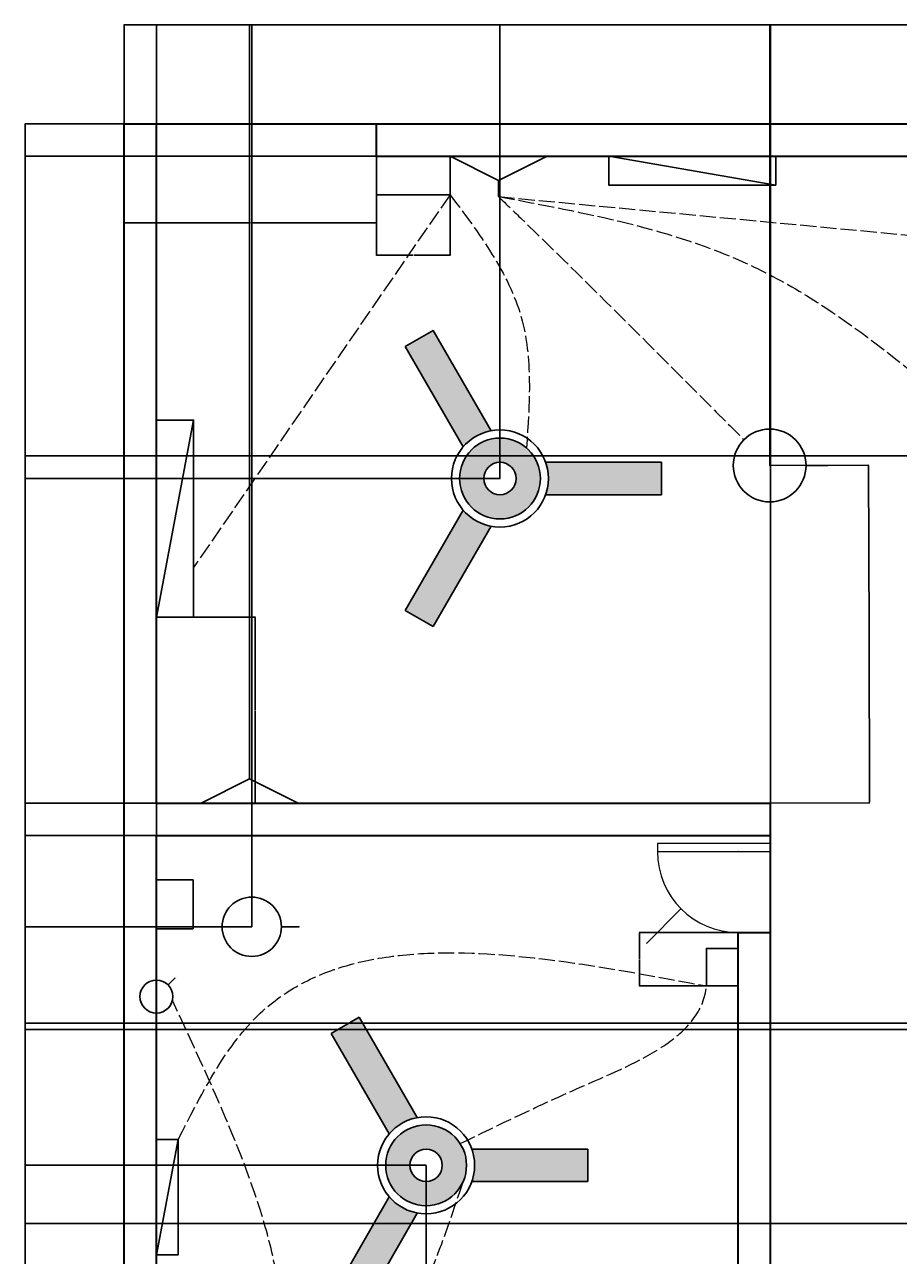
# Model space of a CAD drawing. Units: inches. Extents: x 2034 to 3646, y 962 to 2549.
# Tile 2 of 4: x 2034 to 2683, y 1636 to 2549. Entities that reach past the tile are written whole.
import ezdxf

# ---------------------------------------------------------------- set-up
doc = ezdxf.new("R2010")
doc.units = ezdxf.units.IN
doc.linetypes.add('ACAD_ISO02W100', pattern=[15, 12, -3])
for name, color, linetype, lineweight in [('A-ANNO-DIMS', 2, 'Continuous', 18), ('E-EQPM-FANS', 7, 'Continuous', 30), ('E-LITE-CTRL', 7, 'Continuous', 25), ('E-LITE-FIXT', 7, 'Continuous', 25), ('E-POWR-DEVC', 7, 'Continuous', 25)]:
    doc.layers.add(name, color=color, linetype=linetype, lineweight=lineweight)
for name, color, linetype, lineweight, true_color in [('A-DOOR', 203, 'Continuous', 18, 0xa780c2), ('A-WALL', 203, 'Continuous', 35, 0xa780c2), ('E-LITE-WIRE', 103, 'ACAD_ISO02W100', 18, 0x6dc08b)]:
    doc.layers.add(name, color=color, linetype=linetype, lineweight=lineweight, true_color=true_color)
doc.styles.get("Standard").update_dxf_attribs({"font": 'arial.ttf'})
doc.dimstyles.get("Standard").update_dxf_attribs({"dimtxt": 0.18, "dimasz": 0.18, "dimexe": 0.18, "dimexo": 0.0625, "dimgap": 0.09, "dimtad": 0, "dimtih": 1, "dimtoh": 1, "dimdec": 4, "dimzin": 0, "dimdsep": 46, "dimtxsty": 'Standard', "dimcen": 0.09, "dimadec": 0, "dimazin": 0, "dimtfac": 1, "dimtdec": 4, "dimtofl": 0, "dimtmove": 0, "dimatfit": 3, "dimfxl": 1, "dimtolj": 1, "dimtzin": 0, "dimarcsym": 0})

# ---------------------------------------------------------------- blocks, each defined once
blk = doc.blocks.new('CEILING-FAN-3-BLADE')
h = blk.add_hatch(color=256)
h.dxf.hatch_style = 1
h.paths.add_polyline_path([(-49.61, 109.92), (-70.39, 97.92), (-27.36, 23.39, -0.171573), (-6.58, 35.39)])
h = blk.add_hatch(color=256)
h.dxf.hatch_style = 1
h.paths.add_polyline_path([(-30, 0, 1), (30, 0, 1)])
h.paths.add_polyline_path([(12, 0, -1), (-12, 0, -1)], flags=16)
h = blk.add_hatch(color=256)
h.dxf.hatch_style = 1
h.paths.add_polyline_path([(120, 12), (33.94, 12, -0.085164), (36, 0, -0.085164), (33.94, -12), (120, -12)])
h = blk.add_hatch(color=256)
h.dxf.hatch_style = 1
h.paths.add_polyline_path([(-6.58, -35.39, -0.171573), (-27.36, -23.39), (-70.39, -97.92), (-49.61, -109.92)])
for p, q in [((-70.39, 97.92), (-49.61, 109.92)), ((-49.61, 109.92), (-6.58, 35.39)), ((-27.36, 23.39), (-70.39, 97.92)), ((33.94, 12), (120, 12)), ((120, 12), (120, -12)), ((120, -12), (33.94, -12)), ((-70.39, -97.92), (-27.36, -23.39)), ((-6.58, -35.39), (-49.61, -109.92)), ((-49.61, -109.92), (-70.39, -97.92))]:
    blk.add_line(p, q)
for radius in [36, 30, 12]:
    blk.add_circle((0, 0), radius)
blk = doc.blocks.new('WALL-DEVICE-TRIANGLE')
for p, q in [((-36, 0), (36, 0)), ((0, -18), (-36, 0)), ((36, 0), (0, -18)), ((0, -18), (0, -30))]:
    blk.add_line(p, q)
blk = doc.blocks.new('*D4')
at = {"layer": 'A-ANNO-DIMS', "color": 0, "lineweight": -2, "transparency": 16777216}
for p, q in [((2108.2, 2475.7), (2108.2, 2549.27)), ((2108.38, 2549.09), (2839.85, 2549.09)), ((3572.02, 2549.09), (2840.55, 2549.09)), ((3572.2, 2475.7), (3572.2, 2549.27))]:
    blk.add_line(p, q, dxfattribs=at)
at = {"layer": 'A-ANNO-DIMS', "color": 0, "transparency": 16777216}
for points in [[(2108.38, 2549.12), (2108.38, 2549.06), (2108.2, 2549.09)], [(3572.02, 2549.12), (3572.02, 2549.06), (3572.2, 2549.09)]]:
    blk.add_solid(points, dxfattribs=at)
at = {"layer": 'Defpoints', "color": 0, "transparency": 16777216}
for p in [(3572.2, 2549.09), (2108.2, 2475.64), (3572.2, 2475.64)]:
    blk.add_point(p, dxfattribs=at)
at = {"layer": 'A-ANNO-DIMS', "color": 0, "transparency": 16777216, "insert": (2840.2, 2549.09), "char_height": 0.18, "attachment_point": 5}
blk.add_mtext('\\A1;1464', dxfattribs=at)
blk = doc.blocks.new('*D5')
at = {"layer": 'A-ANNO-DIMS', "color": 0, "lineweight": -2, "transparency": 16777216}
for p, q in [((2108.14, 2475.64), (2034.57, 2475.64)), ((2034.75, 2475.46), (2034.75, 1755.82)), ((2034.75, 1035.82), (2034.75, 1755.46)), ((2682.26, 1035.64), (2034.57, 1035.64))]:
    blk.add_line(p, q, dxfattribs=at)
at = {"layer": 'A-ANNO-DIMS', "color": 0, "transparency": 16777216}
for points in [[(2034.72, 2475.46), (2034.78, 2475.46), (2034.75, 2475.64)], [(2034.72, 1035.82), (2034.78, 1035.82), (2034.75, 1035.64)]]:
    blk.add_solid(points, dxfattribs=at)
at = {"layer": 'Defpoints', "color": 0, "transparency": 16777216}
for p in [(2034.75, 2475.64), (2108.2, 2475.64), (2682.32, 1035.64)]:
    blk.add_point(p, dxfattribs=at)
at = {"layer": 'A-ANNO-DIMS', "color": 0, "transparency": 16777216, "insert": (2034.75, 1755.64), "char_height": 0.18, "attachment_point": 5}
blk.add_mtext('\\A1;1440', dxfattribs=at)
blk = doc.blocks.new('*D14')
at = {"layer": 'A-ANNO-DIMS', "color": 0, "lineweight": -2, "transparency": 16777216}
for p, q in [((2132.14, 2451.64), (2034.57, 2451.64)), ((2034.75, 2451.46), (2034.75, 2211.82)), ((2034.75, 1971.82), (2034.75, 2211.46)), ((2132.14, 1971.64), (2034.57, 1971.64))]:
    blk.add_line(p, q, dxfattribs=at)
at = {"layer": 'A-ANNO-DIMS', "color": 0, "transparency": 16777216}
for points in [[(2034.72, 2451.46), (2034.78, 2451.46), (2034.75, 2451.64)], [(2034.72, 1971.82), (2034.78, 1971.82), (2034.75, 1971.64)]]:
    blk.add_solid(points, dxfattribs=at)
at = {"layer": 'Defpoints', "color": 0, "transparency": 16777216}
for p in [(2034.75, 2451.64), (2132.2, 2451.64), (2132.2, 1971.64)]:
    blk.add_point(p, dxfattribs=at)
at = {"layer": 'A-ANNO-DIMS', "color": 0, "transparency": 16777216, "insert": (2034.75, 2211.64), "char_height": 0.18, "attachment_point": 5}
blk.add_mtext('\\A1;480', dxfattribs=at)
blk = doc.blocks.new('*D15')
at = {"layer": 'A-ANNO-DIMS', "color": 0, "lineweight": -2, "transparency": 16777216}
for p, q in [((2588.2, 1971.7), (2588.2, 2549.27)), ((2588.38, 2549.09), (2705.7, 2549.09)), ((2823.95, 2549.09), (2706.63, 2549.09)), ((2824.13, 1971.7), (2824.13, 2549.27))]:
    blk.add_line(p, q, dxfattribs=at)
at = {"layer": 'A-ANNO-DIMS', "color": 0, "transparency": 16777216}
for points in [[(2588.38, 2549.12), (2588.38, 2549.06), (2588.2, 2549.09)], [(2823.95, 2549.12), (2823.95, 2549.06), (2824.13, 2549.09)]]:
    blk.add_solid(points, dxfattribs=at)
at = {"layer": 'Defpoints', "color": 0, "transparency": 16777216}
for p in [(2824.13, 2549.09), (2588.2, 1971.64), (2824.13, 1971.64)]:
    blk.add_point(p, dxfattribs=at)
at = {"layer": 'A-ANNO-DIMS', "color": 0, "transparency": 16777216, "insert": (2706.16, 2549.09), "char_height": 0.18, "attachment_point": 5}
blk.add_mtext('\\A1;235.93', dxfattribs=at)
blk = doc.blocks.new('*D16')
at = {"layer": 'A-ANNO-DIMS', "color": 0, "lineweight": -2, "transparency": 16777216}
for p, q in [((2588.2, 1635.7), (2588.2, 2549.27)), ((2588.38, 2549.09), (2935.91, 2549.09)), ((3284.02, 2549.09), (2936.49, 2549.09)), ((3284.2, 1635.7), (3284.2, 2549.27))]:
    blk.add_line(p, q, dxfattribs=at)
at = {"layer": 'A-ANNO-DIMS', "color": 0, "transparency": 16777216}
for points in [[(2588.38, 2549.12), (2588.38, 2549.06), (2588.2, 2549.09)], [(3284.02, 2549.12), (3284.02, 2549.06), (3284.2, 2549.09)]]:
    blk.add_solid(points, dxfattribs=at)
at = {"layer": 'Defpoints', "color": 0, "transparency": 16777216}
for p in [(3284.2, 2549.09), (2588.2, 1635.64), (3284.2, 1635.64)]:
    blk.add_point(p, dxfattribs=at)
at = {"layer": 'A-ANNO-DIMS', "color": 0, "transparency": 16777216, "insert": (2936.2, 2549.09), "char_height": 0.18, "attachment_point": 5}
blk.add_mtext('\\A1;696', dxfattribs=at)
blk = doc.blocks.new('*D20')
at = {"layer": 'A-ANNO-DIMS', "color": 0, "lineweight": -2, "transparency": 16777216}
for p, q in [((3300.28, 1803.64), (2034.57, 1803.64)), ((2034.75, 1803.46), (2034.75, 1731.82)), ((2034.75, 1659.82), (2034.75, 1731.46)), ((3300.28, 1659.64), (2034.57, 1659.64))]:
    blk.add_line(p, q, dxfattribs=at)
at = {"layer": 'A-ANNO-DIMS', "color": 0, "transparency": 16777216}
for points in [[(2034.72, 1803.46), (2034.78, 1803.46), (2034.75, 1803.64)], [(2034.72, 1659.82), (2034.78, 1659.82), (2034.75, 1659.64)]]:
    blk.add_solid(points, dxfattribs=at)
at = {"layer": 'Defpoints', "color": 0, "transparency": 16777216}
for p in [(2034.75, 1803.64), (3300.34, 1803.64), (3300.34, 1659.64)]:
    blk.add_point(p, dxfattribs=at)
at = {"layer": 'A-ANNO-DIMS', "color": 0, "transparency": 16777216, "insert": (2034.75, 1731.64), "char_height": 0.18, "attachment_point": 5}
blk.add_mtext('\\A1;144', dxfattribs=at)
blk = doc.blocks.new('*D24')
at = {"layer": 'A-ANNO-DIMS', "color": 0, "lineweight": -2, "transparency": 16777216}
for p, q in [((2132.2, 2255.92), (2132.2, 2549.27)), ((2132.38, 2549.09), (2259.25, 2549.09)), ((2387.05, 2549.09), (2260.18, 2549.09)), ((2387.23, 2212.56), (2387.23, 2549.27))]:
    blk.add_line(p, q, dxfattribs=at)
at = {"layer": 'A-ANNO-DIMS', "color": 0, "transparency": 16777216}
for points in [[(2132.38, 2549.12), (2132.38, 2549.06), (2132.2, 2549.09)], [(2387.05, 2549.12), (2387.05, 2549.06), (2387.23, 2549.09)]]:
    blk.add_solid(points, dxfattribs=at)
at = {"layer": 'Defpoints', "color": 0, "transparency": 16777216}
for p in [(2387.23, 2549.09), (2132.2, 2255.85), (2387.23, 2212.5)]:
    blk.add_point(p, dxfattribs=at)
at = {"layer": 'A-ANNO-DIMS', "color": 0, "transparency": 16777216, "insert": (2259.71, 2549.09), "char_height": 0.18, "attachment_point": 5}
blk.add_mtext('\\A1;255.03', dxfattribs=at)
blk = doc.blocks.new('*D25')
at = {"layer": 'A-ANNO-DIMS', "color": 0, "lineweight": -2, "transparency": 16777216}
for p, q in [((2387.23, 2212.56), (2387.23, 2549.27)), ((2387.41, 2549.09), (2486.88, 2549.09)), ((2587.29, 2549.09), (2487.81, 2549.09)), ((2587.47, 2222.22), (2587.47, 2549.27))]:
    blk.add_line(p, q, dxfattribs=at)
at = {"layer": 'A-ANNO-DIMS', "color": 0, "transparency": 16777216}
for points in [[(2387.41, 2549.12), (2387.41, 2549.06), (2387.23, 2549.09)], [(2587.29, 2549.12), (2587.29, 2549.06), (2587.47, 2549.09)]]:
    blk.add_solid(points, dxfattribs=at)
at = {"layer": 'Defpoints', "color": 0, "transparency": 16777216}
for p in [(2587.47, 2549.09), (2587.47, 2222.15), (2387.23, 2212.5)]:
    blk.add_point(p, dxfattribs=at)
at = {"layer": 'A-ANNO-DIMS', "color": 0, "transparency": 16777216, "insert": (2487.35, 2549.09), "char_height": 0.18, "attachment_point": 5}
blk.add_mtext('\\A1;200.24', dxfattribs=at)
blk = doc.blocks.new('*D26')
at = {"layer": 'A-ANNO-DIMS', "color": 0, "lineweight": -2, "transparency": 16777216}
for p, q in [((2587.47, 2222.22), (2587.47, 2549.27)), ((2587.65, 2549.09), (2679.2, 2549.09)), ((2771.3, 2549.09), (2679.76, 2549.09)), ((2771.48, 2229.49), (2771.48, 2549.27))]:
    blk.add_line(p, q, dxfattribs=at)
at = {"layer": 'A-ANNO-DIMS', "color": 0, "transparency": 16777216}
for points in [[(2587.65, 2549.12), (2587.65, 2549.06), (2587.47, 2549.09)], [(2771.3, 2549.12), (2771.3, 2549.06), (2771.48, 2549.09)]]:
    blk.add_solid(points, dxfattribs=at)
at = {"layer": 'Defpoints', "color": 0, "transparency": 16777216}
for p in [(2771.48, 2549.09), (2771.48, 2229.42), (2587.47, 2222.15)]:
    blk.add_point(p, dxfattribs=at)
at = {"layer": 'A-ANNO-DIMS', "color": 0, "transparency": 16777216, "insert": (2679.48, 2549.09), "char_height": 0.18, "attachment_point": 5}
blk.add_mtext('\\A1;184', dxfattribs=at)
blk = doc.blocks.new('*D27')
at = {"layer": 'A-ANNO-DIMS', "color": 0, "lineweight": -2, "transparency": 16777216}
for p, q in [((2387.17, 2212.5), (2034.57, 2212.5)), ((2034.75, 2212.32), (2034.75, 2092.25)), ((2034.75, 1971.82), (2034.75, 2091.89)), ((2132.14, 1971.64), (2034.57, 1971.64))]:
    blk.add_line(p, q, dxfattribs=at)
at = {"layer": 'A-ANNO-DIMS', "color": 0, "transparency": 16777216}
for points in [[(2034.72, 2212.32), (2034.78, 2212.32), (2034.75, 2212.5)], [(2034.72, 1971.82), (2034.78, 1971.82), (2034.75, 1971.64)]]:
    blk.add_solid(points, dxfattribs=at)
at = {"layer": 'Defpoints', "color": 0, "transparency": 16777216}
for p in [(2034.75, 2212.5), (2387.23, 2212.5), (2132.2, 1971.64)]:
    blk.add_point(p, dxfattribs=at)
at = {"layer": 'A-ANNO-DIMS', "color": 0, "transparency": 16777216, "insert": (2034.75, 2092.07), "char_height": 0.18, "attachment_point": 5}
blk.add_mtext('\\A1;240.86', dxfattribs=at)
blk = doc.blocks.new('*D28')
at = {"layer": 'A-ANNO-DIMS', "color": 0, "lineweight": -2, "transparency": 16777216}
for p, q in [((2785.69, 2451.64), (2034.57, 2451.64)), ((2034.75, 2451.46), (2034.75, 2340.71)), ((2034.75, 2229.6), (2034.75, 2340.35)), ((2771.42, 2229.42), (2034.57, 2229.42))]:
    blk.add_line(p, q, dxfattribs=at)
at = {"layer": 'A-ANNO-DIMS', "color": 0, "transparency": 16777216}
for points in [[(2034.72, 2451.46), (2034.78, 2451.46), (2034.75, 2451.64)], [(2034.72, 2229.6), (2034.78, 2229.6), (2034.75, 2229.42)]]:
    blk.add_solid(points, dxfattribs=at)
at = {"layer": 'Defpoints', "color": 0, "transparency": 16777216}
for p in [(2034.75, 2451.64), (2785.75, 2451.64), (2771.48, 2229.42)]:
    blk.add_point(p, dxfattribs=at)
at = {"layer": 'A-ANNO-DIMS', "color": 0, "transparency": 16777216, "insert": (2034.75, 2340.53), "char_height": 0.18, "attachment_point": 5}
blk.add_mtext('\\A1;222.2', dxfattribs=at)
blk = doc.blocks.new('*D29')
at = {"layer": 'A-ANNO-DIMS', "color": 0, "lineweight": -2, "transparency": 16777216}
for p, q in [((2587.53, 2222.15), (2661.1, 2222.37)), ((2660.92, 2222.19), (2661.28, 2097.29)), ((2661.65, 1972.03), (2661.28, 2096.93)), ((2588.26, 1971.64), (2661.83, 1971.85))]:
    blk.add_line(p, q, dxfattribs=at)
at = {"layer": 'A-ANNO-DIMS', "color": 0, "transparency": 16777216}
for points in [[(2660.95, 2222.19), (2660.89, 2222.19), (2660.92, 2222.37)], [(2661.68, 1972.03), (2661.62, 1972.03), (2661.65, 1971.85)]]:
    blk.add_solid(points, dxfattribs=at)
at = {"layer": 'Defpoints', "color": 0, "transparency": 16777216}
for p in [(2587.47, 2222.15), (2588.2, 1971.64), (2661.65, 1971.85)]:
    blk.add_point(p, dxfattribs=at)
at = {"layer": 'A-ANNO-DIMS', "color": 0, "transparency": 16777216, "insert": (2661.28, 2097.11), "char_height": 0.18, "attachment_point": 5}
blk.add_mtext('\\A1;250.5', dxfattribs=at)
blk = doc.blocks.new('*D30')
at = {"layer": 'A-ANNO-DIMS', "color": 0, "lineweight": -2, "transparency": 16777216}
for p, q in [((2332.44, 1702.82), (2332.44, 962.01)), ((2132.2, 1431.58), (2132.2, 962.01)), ((2132.38, 962.19), (2231.85, 962.19)), ((2332.26, 962.19), (2232.78, 962.19))]:
    blk.add_line(p, q, dxfattribs=at)
at = {"layer": 'A-ANNO-DIMS', "color": 0, "transparency": 16777216}
for points in [[(2132.38, 962.22), (2132.38, 962.16), (2132.2, 962.19)], [(2332.26, 962.22), (2332.26, 962.16), (2332.44, 962.19)]]:
    blk.add_solid(points, dxfattribs=at)
at = {"layer": 'Defpoints', "color": 0, "transparency": 16777216}
for p in [(2332.44, 1702.88), (2132.2, 1431.64), (2332.44, 962.19)]:
    blk.add_point(p, dxfattribs=at)
at = {"layer": 'A-ANNO-DIMS', "color": 0, "transparency": 16777216, "insert": (2232.32, 962.19), "char_height": 0.18, "attachment_point": 5}
blk.add_mtext('\\A1;200.24', dxfattribs=at)
blk = doc.blocks.new('*D31')
at = {"layer": 'A-ANNO-DIMS', "color": 0, "lineweight": -2, "transparency": 16777216}
for p, q in [((2332.38, 1702.88), (2034.57, 1702.88)), ((2034.75, 1702.7), (2034.75, 1567.44)), ((2034.75, 1431.82), (2034.75, 1567.08)), ((2132.14, 1431.64), (2034.57, 1431.64))]:
    blk.add_line(p, q, dxfattribs=at)
at = {"layer": 'A-ANNO-DIMS', "color": 0, "transparency": 16777216}
for points in [[(2034.72, 1702.7), (2034.78, 1702.7), (2034.75, 1702.88)], [(2034.72, 1431.82), (2034.78, 1431.82), (2034.75, 1431.64)]]:
    blk.add_solid(points, dxfattribs=at)
at = {"layer": 'Defpoints', "color": 0, "transparency": 16777216}
for p in [(2034.75, 1702.88), (2332.44, 1702.88), (2132.2, 1431.64)]:
    blk.add_point(p, dxfattribs=at)
at = {"layer": 'A-ANNO-DIMS', "color": 0, "transparency": 16777216, "insert": (2034.75, 1567.26), "char_height": 0.18, "attachment_point": 5}
blk.add_mtext('\\A1;271.24', dxfattribs=at)
blk = doc.blocks.new('*D32')
at = {"layer": 'A-ANNO-DIMS', "color": 0, "lineweight": -2, "transparency": 16777216}
for p, q in [((2132.14, 1947.64), (2034.57, 1947.64)), ((2034.75, 1947.46), (2034.75, 1913.94)), ((2034.75, 1880.05), (2034.75, 1913.57)), ((2202.93, 1879.87), (2034.57, 1879.87))]:
    blk.add_line(p, q, dxfattribs=at)
at = {"layer": 'A-ANNO-DIMS', "color": 0, "transparency": 16777216}
for points in [[(2034.72, 1947.46), (2034.78, 1947.46), (2034.75, 1947.64)], [(2034.72, 1880.05), (2034.78, 1880.05), (2034.75, 1879.87)]]:
    blk.add_solid(points, dxfattribs=at)
at = {"layer": 'Defpoints', "color": 0, "transparency": 16777216}
for p in [(2034.75, 1947.64), (2132.2, 1947.64), (2203, 1879.87)]:
    blk.add_point(p, dxfattribs=at)
at = {"layer": 'A-ANNO-DIMS', "color": 0, "transparency": 16777216, "insert": (2034.75, 1913.76), "char_height": 0.18, "attachment_point": 5}
blk.add_mtext('\\A1;67.77', dxfattribs=at)
blk = doc.blocks.new('*D40')
at = {"layer": 'A-ANNO-DIMS', "color": 0, "lineweight": -2, "transparency": 16777216}
for p, q in [((2108.2, 2475.58), (2108.2, 2402.01)), ((2295.5, 2475.58), (2295.5, 2402.01)), ((2108.38, 2402.19), (2201.46, 2402.19)), ((2295.32, 2402.19), (2202.23, 2402.19))]:
    blk.add_line(p, q, dxfattribs=at)
at = {"layer": 'A-ANNO-DIMS', "color": 0, "transparency": 16777216}
for points in [[(2108.38, 2402.22), (2108.38, 2402.16), (2108.2, 2402.19)], [(2295.32, 2402.22), (2295.32, 2402.16), (2295.5, 2402.19)]]:
    blk.add_solid(points, dxfattribs=at)
at = {"layer": 'Defpoints', "color": 0, "transparency": 16777216}
for p in [(2108.2, 2475.64), (2295.5, 2475.64), (2108.2, 2402.19)]:
    blk.add_point(p, dxfattribs=at)
at = {"layer": 'A-ANNO-DIMS', "color": 0, "transparency": 16777216, "insert": (2201.85, 2402.19), "char_height": 0.18, "attachment_point": 5}
blk.add_mtext('\\A1;187.3', dxfattribs=at)
blk = doc.blocks.new('*D41')
at = {"layer": 'A-ANNO-DIMS', "color": 0, "lineweight": -2, "transparency": 16777216}
for p, q in [((2295.5, 2451.58), (2295.5, 2378.01)), ((2350.19, 2451.58), (2350.19, 2378.01)), ((2295.68, 2378.19), (2322.45, 2378.19)), ((2350.01, 2378.19), (2323.24, 2378.19))]:
    blk.add_line(p, q, dxfattribs=at)
at = {"layer": 'A-ANNO-DIMS', "color": 0, "transparency": 16777216}
for points in [[(2295.68, 2378.22), (2295.68, 2378.16), (2295.5, 2378.19)], [(2350.01, 2378.22), (2350.01, 2378.16), (2350.19, 2378.19)]]:
    blk.add_solid(points, dxfattribs=at)
at = {"layer": 'Defpoints', "color": 0, "transparency": 16777216}
for p in [(2295.5, 2451.64), (2350.19, 2451.64), (2295.5, 2378.19)]:
    blk.add_point(p, dxfattribs=at)
at = {"layer": 'A-ANNO-DIMS', "color": 0, "transparency": 16777216, "insert": (2322.84, 2378.19), "char_height": 0.18, "attachment_point": 5}
blk.add_mtext('\\A1;54.69', dxfattribs=at)
blk = doc.blocks.new('*D42')
at = {"layer": 'A-ANNO-DIMS', "color": 0, "lineweight": -2, "transparency": 16777216}
for p, q in [((2132.2, 1971.7), (2132.2, 2549.27)), ((2132.38, 2549.09), (2166.39, 2549.09)), ((2201.19, 2549.09), (2167.18, 2549.09)), ((2201.37, 1989.7), (2201.37, 2549.27))]:
    blk.add_line(p, q, dxfattribs=at)
at = {"layer": 'A-ANNO-DIMS', "color": 0, "transparency": 16777216}
for points in [[(2132.38, 2549.12), (2132.38, 2549.06), (2132.2, 2549.09)], [(2201.19, 2549.12), (2201.19, 2549.06), (2201.37, 2549.09)]]:
    blk.add_solid(points, dxfattribs=at)
at = {"layer": 'Defpoints', "color": 0, "transparency": 16777216}
for p in [(2201.37, 2549.09), (2201.37, 1989.64), (2132.2, 1971.64)]:
    blk.add_point(p, dxfattribs=at)
at = {"layer": 'A-ANNO-DIMS', "color": 0, "transparency": 16777216, "insert": (2166.78, 2549.09), "char_height": 0.18, "attachment_point": 5}
blk.add_mtext('\\A1;69.17', dxfattribs=at)
blk = doc.blocks.new('*D43')
at = {"layer": 'A-ANNO-DIMS', "color": 0, "lineweight": -2, "transparency": 16777216}
for p, q in [((2132.2, 1947.7), (2132.2, 2549.27)), ((2132.38, 2549.09), (2167.27, 2549.09)), ((2202.82, 2549.09), (2167.92, 2549.09)), ((2203, 1879.94), (2203, 2549.27))]:
    blk.add_line(p, q, dxfattribs=at)
at = {"layer": 'A-ANNO-DIMS', "color": 0, "transparency": 16777216}
for points in [[(2132.38, 2549.12), (2132.38, 2549.06), (2132.2, 2549.09)], [(2202.82, 2549.12), (2202.82, 2549.06), (2203, 2549.09)]]:
    blk.add_solid(points, dxfattribs=at)
at = {"layer": 'Defpoints', "color": 0, "transparency": 16777216}
for p in [(2203, 2549.09), (2132.2, 1947.64), (2203, 1879.87)]:
    blk.add_point(p, dxfattribs=at)
at = {"layer": 'A-ANNO-DIMS', "color": 0, "transparency": 16777216, "insert": (2167.6, 2549.09), "char_height": 0.18, "attachment_point": 5}
blk.add_mtext('\\A1;70.8', dxfattribs=at)
blk = doc.blocks.new('*D44')
at = {"layer": 'A-ANNO-DIMS', "color": 0, "lineweight": -2, "transparency": 16777216}
for p, q in [((2202.93, 1879.87), (2034.57, 1879.87)), ((2034.75, 1879.69), (2034.75, 1791.56)), ((2034.75, 1703.06), (2034.75, 1791.2)), ((2332.38, 1702.88), (2034.57, 1702.88))]:
    blk.add_line(p, q, dxfattribs=at)
at = {"layer": 'A-ANNO-DIMS', "color": 0, "transparency": 16777216}
for points in [[(2034.72, 1879.69), (2034.78, 1879.69), (2034.75, 1879.87)], [(2034.72, 1703.06), (2034.78, 1703.06), (2034.75, 1702.88)]]:
    blk.add_solid(points, dxfattribs=at)
at = {"layer": 'Defpoints', "color": 0, "transparency": 16777216}
for p in [(2034.75, 1879.87), (2203, 1879.87), (2332.44, 1702.88)]:
    blk.add_point(p, dxfattribs=at)
at = {"layer": 'A-ANNO-DIMS', "color": 0, "transparency": 16777216, "insert": (2034.75, 1791.38), "char_height": 0.18, "attachment_point": 5}
blk.add_mtext('\\A1;177', dxfattribs=at)
blk = doc.blocks.new('*D45')
at = {"layer": 'A-ANNO-DIMS', "color": 0, "lineweight": -2, "transparency": 16777216}
for p, q in [((2701.68, 1808.27), (2034.57, 1808.27)), ((2034.75, 1808.09), (2034.75, 1734.14)), ((2034.75, 1659.82), (2034.75, 1733.77)), ((2802.36, 1659.64), (2034.57, 1659.64))]:
    blk.add_line(p, q, dxfattribs=at)
at = {"layer": 'A-ANNO-DIMS', "color": 0, "transparency": 16777216}
for points in [[(2034.72, 1808.09), (2034.78, 1808.09), (2034.75, 1808.27)], [(2034.72, 1659.82), (2034.78, 1659.82), (2034.75, 1659.64)]]:
    blk.add_solid(points, dxfattribs=at)
at = {"layer": 'Defpoints', "color": 0, "transparency": 16777216}
for p in [(2034.75, 1808.27), (2701.74, 1808.27), (2802.42, 1659.64)]:
    blk.add_point(p, dxfattribs=at)
at = {"layer": 'A-ANNO-DIMS', "color": 0, "transparency": 16777216, "insert": (2034.75, 1733.96), "char_height": 0.18, "attachment_point": 5}
blk.add_mtext('\\A1;148.63', dxfattribs=at)
blk = doc.blocks.new('*D55')
at = {"layer": 'A-ANNO-DIMS', "color": 0, "lineweight": -2, "transparency": 16777216}
for p, q in [((2132.26, 2109.51), (2205.83, 2109.51)), ((2205.65, 2109.33), (2205.65, 2040.76)), ((2205.65, 1971.82), (2205.65, 2040.39)), ((2132.26, 1971.64), (2205.83, 1971.64))]:
    blk.add_line(p, q, dxfattribs=at)
at = {"layer": 'A-ANNO-DIMS', "color": 0, "transparency": 16777216}
for points in [[(2205.62, 2109.33), (2205.68, 2109.33), (2205.65, 2109.51)], [(2205.62, 1971.82), (2205.68, 1971.82), (2205.65, 1971.64)]]:
    blk.add_solid(points, dxfattribs=at)
at = {"layer": 'Defpoints', "color": 0, "transparency": 16777216}
for p in [(2132.2, 2109.51), (2132.2, 1971.64), (2205.65, 1971.64)]:
    blk.add_point(p, dxfattribs=at)
at = {"layer": 'A-ANNO-DIMS', "color": 0, "transparency": 16777216, "insert": (2205.65, 2040.58), "char_height": 0.18, "attachment_point": 5}
blk.add_mtext('\\A1;137.87', dxfattribs=at)
blk = doc.blocks.new('*D57')
at = {"layer": 'A-ANNO-DIMS', "color": 0, "lineweight": -2, "transparency": 16777216}
for p, q in [((2564.14, 1875.64), (2490.57, 1875.64)), ((2490.75, 1875.46), (2490.75, 1855.98)), ((2490.75, 1836.13), (2490.75, 1855.61)), ((2564.14, 1835.95), (2490.57, 1835.95))]:
    blk.add_line(p, q, dxfattribs=at)
at = {"layer": 'A-ANNO-DIMS', "color": 0, "transparency": 16777216}
for points in [[(2490.72, 1875.46), (2490.78, 1875.46), (2490.75, 1875.64)], [(2490.72, 1836.13), (2490.78, 1836.13), (2490.75, 1835.95)]]:
    blk.add_solid(points, dxfattribs=at)
at = {"layer": 'Defpoints', "color": 0, "transparency": 16777216}
for p in [(2490.75, 1875.64), (2564.2, 1875.64), (2564.2, 1835.95)]:
    blk.add_point(p, dxfattribs=at)
at = {"layer": 'A-ANNO-DIMS', "color": 0, "transparency": 16777216, "insert": (2490.75, 1855.8), "char_height": 0.18, "attachment_point": 5}
blk.add_mtext('\\A1;39.69', dxfattribs=at)
blk = doc.blocks.new('*D63')
at = {"layer": 'A-ANNO-DIMS', "color": 0, "lineweight": -2, "transparency": 16777216}
for p, q in [((2564.11, 1935.64), (2564.29, 1935.64)), ((2564.2, 1935.55), (2564.2, 1935.73)), ((2496.32, 1867.76), (2521.64, 1893.09)), ((2496.14, 1867.76), (2496.32, 1867.76))]:
    blk.add_line(p, q, dxfattribs=at)
at = {"layer": 'A-ANNO-DIMS', "color": 0, "transparency": 16777216}
blk.add_solid([(2521.62, 1893.11), (2521.67, 1893.06), (2521.77, 1893.21)], dxfattribs=at)
at = {"layer": 'Defpoints', "color": 0, "transparency": 16777216}
for p in [(2564.2, 1935.64), (2521.77, 1893.21)]:
    blk.add_point(p, dxfattribs=at)
at = {"layer": 'A-ANNO-DIMS', "color": 0, "transparency": 16777216, "insert": (2495.83, 1867.76), "char_height": 0.18, "attachment_point": 5}
blk.add_mtext('\\A1;R60', dxfattribs=at)
blk = doc.blocks.new('*D66')
at = {"layer": 'A-ANNO-DIMS', "color": 0, "lineweight": -2, "transparency": 16777216}
for p, q in [((2368.03, 2212.5), (2375.05, 2212.5)), ((2387.14, 2212.5), (2387.32, 2212.5)), ((2387.23, 2212.41), (2387.23, 2212.59))]:
    blk.add_line(p, q, dxfattribs=at)
at = {"layer": 'A-ANNO-DIMS', "color": 0, "transparency": 16777216}
blk.add_solid([(2375.05, 2212.53), (2375.05, 2212.47), (2375.23, 2212.5)], dxfattribs=at)
at = {"layer": 'Defpoints', "color": 0, "transparency": 16777216}
for p in [(2375.23, 2212.5), (2399.23, 2212.49)]:
    blk.add_point(p, dxfattribs=at)
at = {"layer": 'A-ANNO-DIMS', "color": 0, "transparency": 16777216, "insert": (2367.52, 2212.5), "char_height": 0.18, "attachment_point": 5}
blk.add_mtext('\\A1;4X ∅24', dxfattribs=at)
blk = doc.blocks.new('*D67')
at = {"layer": 'A-ANNO-DIMS', "color": 0, "lineweight": -2, "transparency": 16777216}
for p, q in [((2587.38, 2222.15), (2587.56, 2222.15)), ((2587.47, 2222.06), (2587.47, 2222.24)), ((2630.67, 2222.15), (2614.65, 2222.15))]:
    blk.add_line(p, q, dxfattribs=at)
at = {"layer": 'A-ANNO-DIMS', "color": 0, "transparency": 16777216}
blk.add_solid([(2614.65, 2222.18), (2614.65, 2222.12), (2614.47, 2222.15)], dxfattribs=at)
at = {"layer": 'Defpoints', "color": 0, "transparency": 16777216}
for p in [(2560.47, 2222.15), (2614.47, 2222.15)]:
    blk.add_point(p, dxfattribs=at)
at = {"layer": 'A-ANNO-DIMS', "color": 0, "transparency": 16777216, "insert": (2630.98, 2222.15), "char_height": 0.18, "attachment_point": 5}
blk.add_mtext('\\A1;∅54', dxfattribs=at)
blk = doc.blocks.new('*D70')
at = {"layer": 'A-ANNO-DIMS', "color": 0, "lineweight": -2, "transparency": 16777216}
for p, q in [((2202.91, 1879.87), (2203.09, 1879.87)), ((2203, 1879.78), (2203, 1879.96)), ((2238.2, 1879.87), (2225.18, 1879.87))]:
    blk.add_line(p, q, dxfattribs=at)
at = {"layer": 'A-ANNO-DIMS', "color": 0, "transparency": 16777216}
blk.add_solid([(2225.18, 1879.9), (2225.18, 1879.84), (2225, 1879.87)], dxfattribs=at)
at = {"layer": 'Defpoints', "color": 0, "transparency": 16777216}
for p in [(2181, 1879.87), (2225, 1879.87)]:
    blk.add_point(p, dxfattribs=at)
at = {"layer": 'A-ANNO-DIMS', "color": 0, "transparency": 16777216, "insert": (2238.51, 1879.87), "char_height": 0.18, "attachment_point": 5}
blk.add_mtext('\\A1;∅44', dxfattribs=at)
blk = doc.blocks.new('*D76')
at = {"layer": 'A-ANNO-DIMS', "color": 0, "lineweight": -2, "transparency": 16777216}
for p, q in [((2146.06, 1841.94), (2140.99, 1836.88)), ((2146.24, 1841.94), (2146.06, 1841.94)), ((2132.11, 1828.1), (2132.29, 1828.1)), ((2132.2, 1828.01), (2132.2, 1828.19))]:
    blk.add_line(p, q, dxfattribs=at)
at = {"layer": 'A-ANNO-DIMS', "color": 0, "transparency": 16777216}
blk.add_solid([(2140.97, 1836.9), (2141.01, 1836.86), (2140.86, 1836.75)], dxfattribs=at)
at = {"layer": 'Defpoints', "color": 0, "transparency": 16777216}
for p in [(2140.86, 1836.75), (2123.53, 1819.45)]:
    blk.add_point(p, dxfattribs=at)
at = {"layer": 'A-ANNO-DIMS', "color": 0, "transparency": 16777216, "insert": (2146.8, 1841.94), "char_height": 0.18, "attachment_point": 5}
blk.add_mtext('\\A1;∅24.487', dxfattribs=at)

msp = doc.modelspace()

# ---------------------------------------------------------------- linework, layer by layer
at = {"layer": 'A-DOOR'}
for p, q in [((2588.1976, 1947.6388), (2588.1976, 1941.6388)), ((2588.1976, 1941.6388), (2504.1976, 1941.6388)), ((2504.1976, 1941.6388), (2504.1976, 1935.6388)), ((2504.1976, 1935.6388), (2588.1976, 1935.6388))]:
    msp.add_line(p, q, dxfattribs=at)
msp.add_arc((2564.1976, 1935.6388), 60, 180, 270, dxfattribs=at)
at = {"layer": 'A-WALL'}
for p, q in [((2132.1976, 2451.6388), (2132.1976, 2475.6388)), ((2295.4968, 2451.6388), (2295.4968, 2475.6388)), ((2132.1976, 1971.6388), (2132.1976, 2451.6388)), ((2295.4968, 2451.6388), (2737.7486, 2451.6388)), ((2132.1976, 1971.6388), (2588.1976, 1971.6388)), ((2588.1976, 1167.6388), (2588.1976, 1971.6388)), ((2132.1976, 1947.6388), (2588.1976, 1947.6388)), ((2132.1976, 1431.6388), (2132.1976, 1947.6388)), ((2564.1976, 1455.6388), (2564.1976, 1875.6388)), ((2564.1976, 1875.6388), (2588.1976, 1875.6388))]:
    msp.add_line(p, q, dxfattribs=at)
msp.add_lwpolyline([(2108.1976, 1407.6388), (2108.1976, 2475.6388), (3308.1976, 2475.6388)], dxfattribs=at)
at = {"layer": 'E-LITE-CTRL'}
for points in [[(2295.4968, 2451.6388), (2350.1907, 2451.6388), (2350.1907, 2423.0805), (2295.4968, 2423.0805)], [(2564.1976, 1863.838), (2540.5401, 1863.838), (2540.5401, 1835.9523), (2564.1976, 1835.9523)]]:
    msp.add_lwpolyline(points, close=True, dxfattribs=at)
at = {"layer": 'E-LITE-FIXT'}
for p, q in [((2467.9567, 2451.6388), (2592.0157, 2430.2666)), ((2159.7597, 2255.8532), (2132.1976, 2109.5115)), ((2132.1976, 1636.487), (2148.4814, 1721.9994))]:
    msp.add_line(p, q, dxfattribs=at)
for points in [[(2592.0157, 2451.6388), (2467.9567, 2451.6388), (2467.9567, 2430.2666), (2592.0157, 2430.2666)], [(2132.1976, 2109.5115), (2159.7597, 2109.5115), (2159.7597, 2255.8532), (2132.1976, 2255.8532)], [(2132.1976, 1636.487), (2148.4814, 1636.487), (2148.4814, 1721.9994), (2132.1976, 1721.9994)]]:
    msp.add_lwpolyline(points, close=True, dxfattribs=at)
for centre, radius in [((2587.4667, 2222.1542), 27), ((2202.995, 1879.873), 22)]:
    msp.add_circle(centre, radius, dxfattribs=at)
at = {"layer": 'E-LITE-WIRE'}
for p, q in [((2350.1907, 2423.0805), (2159.7597, 2146.4606)), ((2386.1907, 2421.6388), (2984.5836, 2365.4191))]:
    msp.add_line(p, q, dxfattribs=at)
for points, knots in [([(2350.1907, 2423.0805), (2371.9987, 2394.0313), (2413.9945, 2338.0909), (2409.259, 2268.5201), (2406.9826, 2235.0766)], [0, 0, 0, 0, 105.06682456, 202.32859005, 202.32859005, 202.32859005, 202.32859005]), ([(2386.1907, 2421.6388), (2391.9757, 2416.0517), (2453.449, 2356.6816), (2513.7159, 2296.0806), (2568.3114, 2241.1825)], [0, 0, 0, 0, 24.12725166, 256.38536373, 256.38536373, 256.38536373, 256.38536373]), ([(2386.1907, 2421.6388), (2450.6467, 2409.6898), (2584.5763, 2384.8618), (2688.3336, 2296.2606), (2742.1558, 2250.3004)], [0, 0, 0, 0, 193.13075599, 401.29592099, 401.29592099, 401.29592099, 401.29592099]), ([(2148.4814, 1721.9994), (2165.118, 1754.7568), (2235.3408, 1893.0258), (2408.4457, 1860.6545), (2540.5401, 1835.9523)], [0, 0, 0, 0, 104.72557502, 442.04729157, 442.04729157, 442.04729157, 442.04729157]), ([(2357.7124, 1719.0441), (2386.5732, 1733.0306), (2448.4628, 1763.0235), (2542.7009, 1800.7887), (2540.7485, 1845.1596), (2540.5401, 1849.8952)], [0, 0, 0, 0, 101.9717416, 218.66957548, 232.612459, 232.612459, 232.612459, 232.612459]), ([(2132.1976, 1431.6388), (2157.638, 1451.201), (2276.6339, 1542.7023), (2202.4164, 1700.7955), (2144.0659, 1825.0897)], [0, 0, 0, 0, 91.4631997, 427.81459201, 427.81459201, 427.81459201, 427.81459201]), ([(2132.1976, 1431.6388), (2198.2305, 1468.9918), (2306.37, 1530.1634), (2344.9098, 1645.8124), (2359.9161, 1690.843)], [0, 0, 0, 0, 217.15653049, 355.62904492, 355.62904492, 355.62904492, 355.62904492])]:
    msp.add_open_spline(points, degree=3, knots=knots, dxfattribs=at)
at = {"layer": 'E-POWR-DEVC'}
msp.add_lwpolyline([(2132.1976, 1914.705), (2159.4203, 1914.705), (2159.4203, 1878.4217), (2132.1976, 1878.4217)], close=True, dxfattribs=at)
msp.add_circle((2132.1976, 1828.0981), 12.2436, dxfattribs=at)

# ---------------------------------------------------------------- block references
at = {"layer": 'E-EQPM-FANS'}
for p in [(2387.2299, 2212.4972), (2332.4379, 1702.8825)]:
    msp.add_blockref('CEILING-FAN-3-BLADE', p, dxfattribs=at)
at = {"layer": 'E-POWR-DEVC'}
msp.add_blockref('WALL-DEVICE-TRIANGLE', (2386.1907, 2451.6388), dxfattribs=at)
at = {"layer": 'E-POWR-DEVC', "rotation": 180}
msp.add_blockref('WALL-DEVICE-TRIANGLE', (2201.3685, 1971.6388), dxfattribs=at)

# ---------------------------------------------------------------- dimensions: what is measured, and where the dimension line sits
at = {"layer": 'A-ANNO-DIMS'}
for base, p1, p2, override, picture, middle in [((3572.1976, 2549.0888), (2108.1976, 2475.6388), (3572.1976, 2475.6388), {"dimdec": 0, "dimlfac": 1, "dimrnd": 0, "dimzin": 0, "dimdsep": 46, "dimlunit": 2}, '*D4', (2840.1976, 2549.0888)), ((2387.2299, 2549.0888), (2132.1976, 2255.8532), (2387.2299, 2212.4972), {"dimdec": 2, "dimlfac": 1, "dimrnd": 0, "dimzin": 0, "dimdsep": 46, "dimlunit": 2}, '*D24', (2259.7138, 2549.0888)), ((2201.3685, 2549.0888), (2132.1976, 1971.6388), (2201.3685, 1989.6388), {"dimdec": 2, "dimlfac": 1, "dimrnd": 0, "dimzin": 0, "dimdsep": 46, "dimlunit": 2}, '*D42', (2166.783, 2549.0888)), ((2202.995, 2549.0888), (2132.1976, 1947.6388), (2202.995, 1879.873), {"dimdec": 1, "dimlfac": 1, "dimrnd": 0, "dimzin": 0, "dimdsep": 46, "dimlunit": 2}, '*D43', (2167.5963, 2549.0888)), ((2587.4667, 2549.0888), (2387.2299, 2212.4972), (2587.4667, 2222.1542), {"dimdec": 2, "dimlfac": 1, "dimrnd": 0, "dimzin": 0, "dimdsep": 46, "dimlunit": 2}, '*D25', (2487.3483, 2549.0888)), ((2771.4839, 2549.0888), (2587.4667, 2222.1542), (2771.4839, 2229.423), {"dimdec": 0, "dimlfac": 1, "dimrnd": 0, "dimzin": 0, "dimdsep": 46, "dimlunit": 2}, '*D26', (2679.4753, 2549.0888)), ((2824.1305, 2549.0888), (2588.1976, 1971.6388), (2824.1305, 1971.6388), {"dimdec": 2, "dimlfac": 1, "dimrnd": 0, "dimzin": 0, "dimdsep": 46, "dimlunit": 2}, '*D15', (2706.1641, 2549.0888)), ((3284.1976, 2549.0888), (2588.1976, 1635.6388), (3284.1976, 1635.6388), {"dimdec": 0, "dimlfac": 1, "dimrnd": 0, "dimzin": 0, "dimdsep": 46, "dimlunit": 2}, '*D16', (2936.1976, 2549.0888)), ((2332.4379, 962.1888), (2132.1976, 1431.6388), (2332.4379, 1702.8825), {"dimdec": 2, "dimlfac": 1, "dimrnd": 0, "dimzin": 0, "dimdsep": 46, "dimlunit": 2}, '*D30', (2232.3178, 962.1888))]:
    dim = msp.add_linear_dim(base=base, p1=p1, p2=p2, dimstyle='Standard', override=override, dxfattribs=at)
    dim.commit()
    dim.dimension.update_dxf_attribs({"geometry": picture, "text_midpoint": middle})
for base, p1, p2, angle, override, picture, middle in [((2034.7476, 2475.6388), (2682.3208, 1035.6388), (2108.1976, 2475.6388), 90, {"dimdec": 0, "dimlfac": 1, "dimrnd": 0, "dimzin": 0, "dimdsep": 46, "dimlunit": 2}, '*D5', (2034.7476, 1755.6388)), ((2108.1976, 2402.1888), (2295.4968, 2475.6388), (2108.1976, 2475.6388), 180, {"dimdec": 1, "dimlfac": 1, "dimrnd": 0, "dimzin": 0, "dimdsep": 46, "dimlunit": 2}, '*D40', (2201.8472, 2402.1888)), ((2034.7476, 2451.6388), (2771.4839, 2229.423), (2785.7486, 2451.6388), 90, {"dimdec": 1, "dimlfac": 1, "dimrnd": 0, "dimzin": 0, "dimdsep": 46, "dimlunit": 2}, '*D28', (2034.7476, 2340.5309)), ((2034.7476, 2451.6388), (2132.1976, 1971.6388), (2132.1976, 2451.6388), 90, {"dimdec": 0, "dimlfac": 1, "dimrnd": 0, "dimzin": 0, "dimdsep": 46, "dimlunit": 2}, '*D14', (2034.7476, 2211.6388)), ((2295.4968, 2378.1888), (2350.1907, 2451.6388), (2295.4968, 2451.6388), 180, {"dimdec": 2, "dimlfac": 1, "dimrnd": 0, "dimzin": 0, "dimdsep": 46, "dimlunit": 2}, '*D41', (2322.8438, 2378.1888)), ((2661.6473, 1971.8531), (2587.4667, 2222.1542), (2588.1976, 1971.6388), 270.1671779, {"dimdec": 1, "dimlfac": 1, "dimrnd": 0, "dimzin": 0, "dimdsep": 46, "dimlunit": 2}, '*D29', (2661.2818, 2097.1108)), ((2034.7476, 2212.4972), (2132.1976, 1971.6388), (2387.2299, 2212.4972), 90, {"dimdec": 2, "dimlfac": 1, "dimrnd": 0, "dimzin": 0, "dimdsep": 46, "dimlunit": 2}, '*D27', (2034.7476, 2092.068)), ((2205.6476, 1971.6388), (2132.1976, 2109.5115), (2132.1976, 1971.6388), 270, {"dimdec": 2, "dimlfac": 1, "dimrnd": 0, "dimzin": 0, "dimdsep": 46, "dimlunit": 2}, '*D55', (2205.6476, 2040.5751)), ((2034.7476, 1947.6388), (2202.995, 1879.873), (2132.1976, 1947.6388), 90, {"dimdec": 2, "dimlfac": 1, "dimrnd": 0, "dimzin": 0, "dimdsep": 46, "dimlunit": 2}, '*D32', (2034.7476, 1913.7559)), ((2034.7476, 1879.873), (2332.4379, 1702.8825), (2202.995, 1879.873), 90, {"dimdec": 0, "dimlfac": 1, "dimrnd": 0, "dimzin": 0, "dimdsep": 46, "dimlunit": 2}, '*D44', (2034.7476, 1791.3777)), ((2490.7476, 1875.6388), (2564.1976, 1835.9523), (2564.1976, 1875.6388), 90, {"dimdec": 2, "dimlfac": 1, "dimrnd": 0, "dimzin": 0, "dimdsep": 46, "dimlunit": 2}, '*D57', (2490.7476, 1855.7955)), ((2034.7476, 1808.2715), (2802.4216, 1659.6388), (2701.738, 1808.2715), 90, {"dimdec": 2, "dimlfac": 1, "dimrnd": 0, "dimzin": 0, "dimdsep": 46, "dimlunit": 2}, '*D45', (2034.7476, 1733.9551)), ((2034.7476, 1803.6388), (3300.3398, 1659.6388), (3300.3398, 1803.6388), 90, {"dimdec": 0, "dimlfac": 1, "dimrnd": 0, "dimzin": 0, "dimdsep": 46, "dimlunit": 2}, '*D20', (2034.7476, 1731.6388)), ((2034.7476, 1702.8825), (2132.1976, 1431.6388), (2332.4379, 1702.8825), 90, {"dimdec": 2, "dimlfac": 1, "dimrnd": 0, "dimzin": 0, "dimdsep": 46, "dimlunit": 2}, '*D31', (2034.7476, 1567.2606))]:
    dim = msp.add_linear_dim(base=base, p1=p1, p2=p2, angle=angle, dimstyle='Standard', override=override, dxfattribs=at)
    dim.commit()
    dim.dimension.update_dxf_attribs({"geometry": picture, "text_midpoint": middle})
for p1, p2, override, picture, middle in [((2560.4667, 2222.1543), (2614.4667, 2222.154), {"dimdec": 0, "dimlfac": 1, "dimrnd": 0, "dimzin": 0, "dimdsep": 46, "dimlunit": 2}, '*D67', (2630.6667, 2222.1539)), ((2180.995, 1879.873), (2224.995, 1879.873), {"dimdec": 0, "dimlfac": 1, "dimrnd": 0, "dimzin": 0, "dimdsep": 46, "dimlunit": 2}, '*D70', (2238.195, 1879.873)), ((2123.5348, 1819.4458), (2140.8604, 1836.7504), {"dimdec": 3, "dimlfac": 1, "dimrnd": 0, "dimzin": 0, "dimdsep": 46, "dimlunit": 2}, '*D76', (2146.7997, 1841.9418))]:
    dim = msp.add_diameter_dim_2p(p1=p1, p2=p2, dimstyle='Standard', override=override, dxfattribs=at)
    dim.commit()
    dim.dimension.update_dxf_attribs({"geometry": picture, "text_midpoint": middle, "dimtype": 163})
dim = msp.add_diameter_dim_2p(p1=(2399.2299, 2212.4945), p2=(2375.2299, 2212.5), text='4X <>', dimstyle='Standard', override={"dimdec": 0, "dimlfac": 1, "dimrnd": 0, "dimzin": 0, "dimdsep": 46, "dimlunit": 2}, dxfattribs=at)
dim.commit()
dim.dimension.update_dxf_attribs({"geometry": '*D66', "text_midpoint": (2368.0299, 2212.5017), "dimtype": 163})
dim = msp.add_radius_dim(center=(2564.1976, 1935.6388), mpoint=(2521.7713, 1893.2123), dimstyle='Standard', override={"dimdec": 0, "dimlfac": 1, "dimrnd": 0, "dimzin": 0, "dimdsep": 46, "dimlunit": 2}, dxfattribs=at)
dim.commit()
dim.dimension.update_dxf_attribs({"geometry": '*D63', "text_midpoint": (2495.8308, 1867.7564), "dimtype": 164})

doc.saveas('drawing.dxf')
